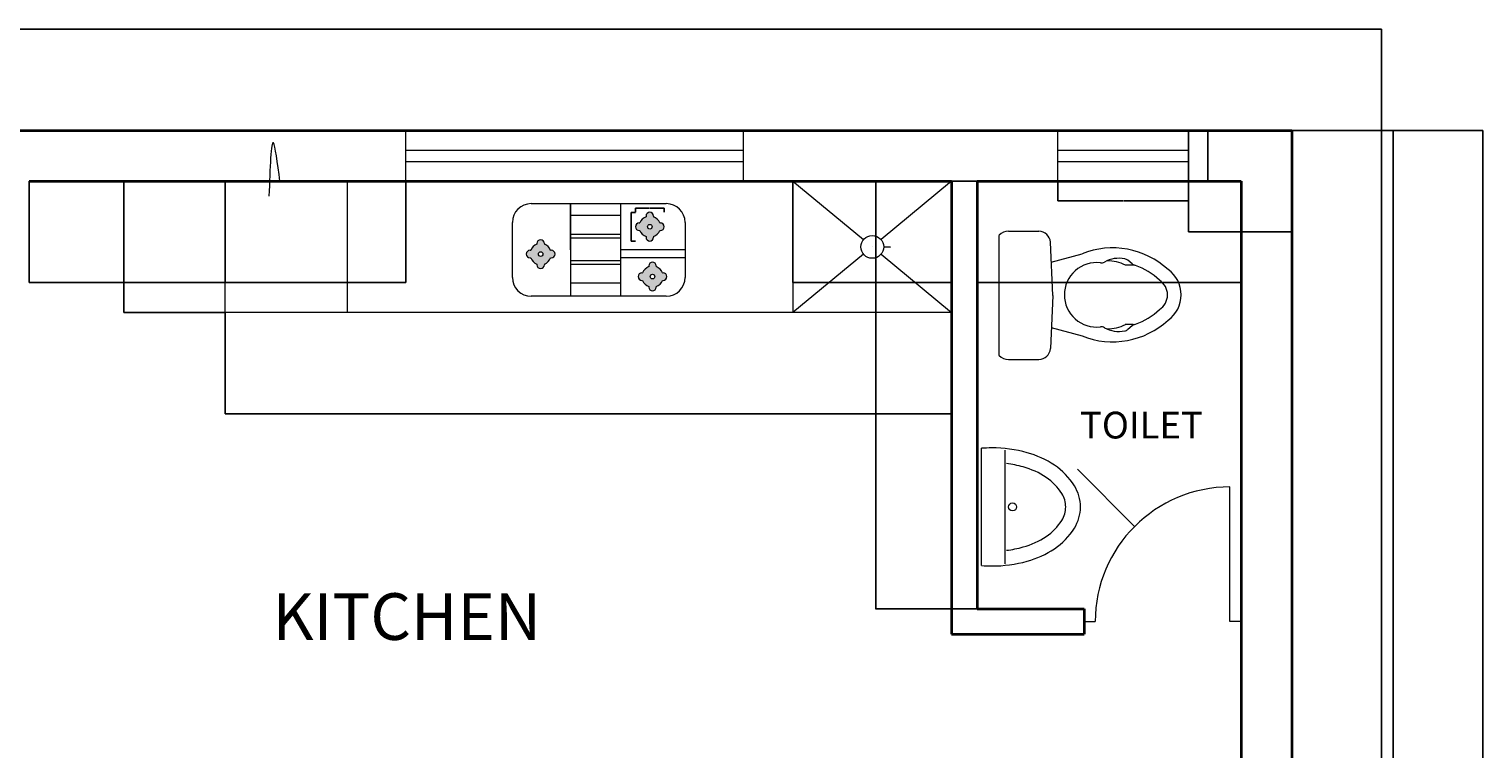
# Model space of a CAD drawing. Units: millimetres. Extents: x 2511 to 24632, y 2213 to 12972.
# Tile 3 of 5: x 6023 to 12605, y 7630 to 10891. Entities that reach past the tile are written whole.
import ezdxf

# ---------------------------------------------------------------- set-up
doc = ezdxf.new("R2010")
doc.units = ezdxf.units.MM
for name, color, linetype, lineweight in [('A-ANNO-DIMS', 2, 'Continuous', 18), ('A-AREA-IDEN', 7, 'Continuous', 20), ('A-EQPM', 4, 'Continuous', 18), ('A-FLOR-CASE', 7, 'Continuous', 18), ('A-FLOR-FIXT', 5, 'Continuous', 18), ('A-WALL', 7, 'Continuous', 35), ('doors', 50, 'Continuous', 18), ('windows', 70, 'Continuous', 18)]:
    doc.layers.add(name, color=color, linetype=linetype, lineweight=lineweight)
doc.styles.get("Standard").update_dxf_attribs({"font": 'arial.ttf'})
doc.dimstyles.get("Standard").update_dxf_attribs({"dimtxt": 0.18, "dimasz": 0.18, "dimexe": 0.18, "dimexo": 0.0625, "dimgap": 0.09, "dimtad": 0, "dimtih": 1, "dimtoh": 1, "dimdec": 4, "dimzin": 0, "dimdsep": 46, "dimtxsty": 'Standard', "dimcen": 0.09, "dimadec": 0, "dimazin": 0, "dimtfac": 1, "dimtdec": 4, "dimtofl": 0, "dimtmove": 0, "dimatfit": 3, "dimfxl": 1, "dimtolj": 1, "dimtzin": 0, "dimarcsym": 0})

# ---------------------------------------------------------------- blocks, each defined once
blk = doc.blocks.new('HOB-BURNER-PLAN')
h = blk.add_hatch(color=256)
h.dxf.hatch_style = 1
h.paths.add_polyline_path([(82.2, 110), (82.2, 113.2, 1), (48.1, 113.2), (48.1, 110, 0.214506), (20.2, 82.2), (17.1, 82.2, 1), (17.1, 48.1), (20.2, 48.1, 0.214506), (48.1, 20.2), (48.1, 17.1, 1), (82.2, 17.1), (82.2, 20.2, 0.214506), (110, 48.1), (113.2, 48.1, 1), (113.2, 82.2), (110, 82.2, 0.214506)])
h.paths.add_polyline_path([(75.5, 65.1, -1), (54.7, 65.1, -1)], flags=16)
for p, q in [((17.1, 82.2), (20.2, 82.2)), ((48.1, 113.2), (48.1, 110)), ((82.2, 113.2), (82.2, 110)), ((110, 82.2), (113.2, 82.2)), ((17.1, 48.1), (20.2, 48.1)), ((48.1, 20.2), (48.1, 17.1)), ((82.2, 20.2), (82.2, 17.1)), ((110, 48.1), (113.2, 48.1))]:
    blk.add_line(p, q)
blk.add_circle((65.1, 65.1), 10.4)
for centre, radius, start, end in [((17.1, 65.1), 17.1, 90, 270), ((65.1, 65.1), 48.1, 110.78637, 159.21363), ((65.1, 113.2), 17.1, 0, 180), ((65.1, 65.1), 48.1, 20.78637, 69.21363), ((113.2, 65.1), 17.1, 270, 90), ((65.1, 65.1), 48.1, 200.78637, 249.21363), ((65.1, 17.1), 17.1, 180, 0), ((65.1, 65.1), 48.1, 290.78637, 339.21363)]:
    blk.add_arc(centre, radius, start, end)
blk = doc.blocks.new('WINDOW-1528-PLAN')
for p, q in [((0, 140), (1528, 140)), ((0, 90), (1528, 90))]:
    blk.add_line(p, q)
blk.add_lwpolyline([(0, 230), (1528, 230), (1528, 0), (0, 0)], close=True)
blk = doc.blocks.new('WINDOW-592-PLAN')
for p, q in [((0, 140), (591.5, 140)), ((0, 90), (591.5, 90))]:
    blk.add_line(p, q)
blk.add_lwpolyline([(0, 230), (591.5, 230), (591.5, 0), (0, 0)], close=True)
blk = doc.blocks.new('*D21')
at = {"layer": 'A-ANNO-DIMS', "color": 0, "lineweight": -2, "transparency": 16777216}
for p, q in [((8768.5, 10060.9), (8768.5, 10080.5)), ((8768.6, 10080.4), (8832.4, 10080.4)), ((8898.5, 10080.4), (8834.7, 10080.4)), ((8898.7, 10060.9), (8898.7, 10080.5))]:
    blk.add_line(p, q, dxfattribs=at)
at = {"layer": 'A-ANNO-DIMS', "color": 0, "transparency": 16777216}
for points in [[(8768.6, 10080.4), (8768.6, 10080.3), (8768.5, 10080.4)], [(8898.5, 10080.4), (8898.5, 10080.3), (8898.7, 10080.4)]]:
    blk.add_solid(points, dxfattribs=at)
at = {"layer": 'Defpoints', "color": 0, "transparency": 16777216}
for p in [(8898.7, 10080.4), (8768.5, 10060.8), (8898.7, 10060.8)]:
    blk.add_point(p, dxfattribs=at)
at = {"layer": 'A-ANNO-DIMS', "color": 0, "transparency": 16777216, "insert": (8833.6, 10080.4), "char_height": 0.18, "attachment_point": 5}
blk.add_mtext('\\A1;BURNER 130 TYP.', dxfattribs=at)
blk = doc.blocks.new('*D22')
at = {"layer": 'A-ANNO-DIMS', "color": 0, "lineweight": -2, "transparency": 16777216}
for p, q in [((8768.4, 10060.8), (8748.7, 10060.8)), ((8748.9, 10060.6), (8748.9, 9995.9)), ((8748.9, 9930.8), (8748.9, 9995.5)), ((8768.4, 9930.6), (8748.7, 9930.6))]:
    blk.add_line(p, q, dxfattribs=at)
at = {"layer": 'A-ANNO-DIMS', "color": 0, "transparency": 16777216}
for points in [[(8748.9, 10060.6), (8749, 10060.6), (8748.9, 10060.8)], [(8748.9, 9930.8), (8749, 9930.8), (8748.9, 9930.6)]]:
    blk.add_solid(points, dxfattribs=at)
at = {"layer": 'Defpoints', "color": 0, "transparency": 16777216}
for p in [(8748.9, 10060.8), (8768.5, 10060.8), (8768.5, 9930.6)]:
    blk.add_point(p, dxfattribs=at)
at = {"layer": 'A-ANNO-DIMS', "color": 0, "transparency": 16777216, "insert": (8748.9, 9995.7), "char_height": 0.18, "attachment_point": 5}
blk.add_mtext('\\A1;130 TYP.', dxfattribs=at)
blk = doc.blocks.new('*D27')
at = {"layer": 'A-ANNO-DIMS', "color": 0, "lineweight": -2, "transparency": 16777216}
for p, q in [((10680.4, 10201.8), (10680.4, 10113)), ((11272, 10201.8), (11272, 10113)), ((10680.6, 10113.1), (10974.8, 10113.1)), ((11271.8, 10113.1), (10977.6, 10113.1))]:
    blk.add_line(p, q, dxfattribs=at)
at = {"layer": 'A-ANNO-DIMS', "color": 0, "transparency": 16777216}
for points in [[(10680.6, 10113.2), (10680.6, 10113.1), (10680.4, 10113.1)], [(11271.8, 10113.2), (11271.8, 10113.1), (11272, 10113.1)]]:
    blk.add_solid(points, dxfattribs=at)
at = {"layer": 'Defpoints', "color": 0, "transparency": 16777216}
for p in [(10680.4, 10201.9), (11272, 10201.9), (11272, 10113.1)]:
    blk.add_point(p, dxfattribs=at)
at = {"layer": 'A-ANNO-DIMS', "color": 0, "transparency": 16777216, "insert": (10976.2, 10113.1), "char_height": 0.18, "attachment_point": 5}
blk.add_mtext('\\A1;WC WINDOW 592 TYP.', dxfattribs=at)
blk = doc.blocks.new('*D28')
at = {"layer": 'A-ANNO-DIMS', "color": 0, "lineweight": -2, "transparency": 16777216}
for p, q in [((11272, 10431.9), (11360.9, 10431.9)), ((11360.7, 10431.7), (11360.7, 10317)), ((11360.7, 10202), (11360.7, 10316.7)), ((11272, 10201.9), (11360.9, 10201.9))]:
    blk.add_line(p, q, dxfattribs=at)
at = {"layer": 'A-ANNO-DIMS', "color": 0, "transparency": 16777216}
for points in [[(11360.7, 10431.7), (11360.7, 10431.7), (11360.7, 10431.9)], [(11360.7, 10202), (11360.7, 10202), (11360.7, 10201.9)]]:
    blk.add_solid(points, dxfattribs=at)
at = {"layer": 'Defpoints', "color": 0, "transparency": 16777216}
for p in [(11272, 10431.9), (11360.7, 10431.9), (11272, 10201.9)]:
    blk.add_point(p, dxfattribs=at)
at = {"layer": 'A-ANNO-DIMS', "color": 0, "transparency": 16777216, "insert": (11360.7, 10316.9), "char_height": 0.18, "attachment_point": 5}
blk.add_mtext('\\A1;230 TYP.', dxfattribs=at)
blk = doc.blocks.new('*D35')
at = {"layer": 'A-ANNO-DIMS', "color": 0, "lineweight": -2, "transparency": 16777216}
for p, q in [((2970.2, 10431.9), (2970.2, 10891)), ((2970.4, 10890.9), (7557.9, 10890.9)), ((12146, 10890.9), (7558.6, 10890.9)), ((12146.2, 7356.9), (12146.2, 10891))]:
    blk.add_line(p, q, dxfattribs=at)
at = {"layer": 'A-ANNO-DIMS', "color": 0, "transparency": 16777216}
for points in [[(2970.4, 10890.9), (2970.4, 10890.8), (2970.2, 10890.9)], [(12146, 10890.9), (12146, 10890.8), (12146.2, 10890.9)]]:
    blk.add_solid(points, dxfattribs=at)
at = {"layer": 'Defpoints', "color": 0, "transparency": 16777216}
for p in [(12146.2, 10890.9), (2970.2, 10431.9), (12146.2, 7356.9)]:
    blk.add_point(p, dxfattribs=at)
at = {"layer": 'A-ANNO-DIMS', "color": 0, "transparency": 16777216, "insert": (7558.2, 10890.9), "char_height": 0.18, "attachment_point": 5}
blk.add_mtext('\\A1;9176', dxfattribs=at)
blk = doc.blocks.new('*D36')
at = {"layer": 'A-ANNO-DIMS', "color": 0, "lineweight": -2, "transparency": 16777216}
for p, q in [((11740.3, 10431.9), (12605.4, 10431.9)), ((12605.2, 10431.7), (12605.2, 6552)), ((12605.2, 2672), (12605.2, 6551.7)), ((9066.3, 2671.9), (12605.4, 2671.9))]:
    blk.add_line(p, q, dxfattribs=at)
at = {"layer": 'A-ANNO-DIMS', "color": 0, "transparency": 16777216}
for points in [[(12605.2, 10431.7), (12605.2, 10431.7), (12605.2, 10431.9)], [(12605.2, 2672), (12605.2, 2672), (12605.2, 2671.9)]]:
    blk.add_solid(points, dxfattribs=at)
at = {"layer": 'Defpoints', "color": 0, "transparency": 16777216}
for p in [(11740.2, 10431.9), (12605.2, 10431.9), (9066.2, 2671.9)]:
    blk.add_point(p, dxfattribs=at)
at = {"layer": 'A-ANNO-DIMS', "color": 0, "transparency": 16777216, "insert": (12605.2, 6551.9), "char_height": 0.18, "attachment_point": 5}
blk.add_mtext('\\A1;7760', dxfattribs=at)
blk = doc.blocks.new('*D50')
at = {"layer": 'A-ANNO-DIMS', "color": 0, "lineweight": -2, "transparency": 16777216}
for p, q in [((6911.1, 9606.7), (6911.1, 9147.6)), ((10200.2, 9606.7), (10200.2, 9147.6)), ((6911.3, 9147.8), (8555.3, 9147.8)), ((10200, 9147.8), (8556, 9147.8))]:
    blk.add_line(p, q, dxfattribs=at)
at = {"layer": 'A-ANNO-DIMS', "color": 0, "transparency": 16777216}
for points in [[(6911.3, 9147.8), (6911.3, 9147.8), (6911.1, 9147.8)], [(10200, 9147.8), (10200, 9147.8), (10200.2, 9147.8)]]:
    blk.add_solid(points, dxfattribs=at)
at = {"layer": 'Defpoints', "color": 0, "transparency": 16777216}
for p in [(6911.1, 9606.8), (10200.2, 9606.8), (6911.1, 9147.8)]:
    blk.add_point(p, dxfattribs=at)
at = {"layer": 'A-ANNO-DIMS', "color": 0, "transparency": 16777216, "insert": (8555.6, 9147.8), "char_height": 0.18, "attachment_point": 5}
blk.add_mtext('\\A1;3289', dxfattribs=at)
blk = doc.blocks.new('*D51')
at = {"layer": 'A-ANNO-DIMS', "color": 0, "lineweight": -2, "transparency": 16777216}
for p, q in [((6911, 10201.9), (6451.9, 10201.9)), ((6452.1, 10201.7), (6452.1, 9904.5)), ((6452.1, 9607), (6452.1, 9904.1)), ((6911, 9606.8), (6451.9, 9606.8))]:
    blk.add_line(p, q, dxfattribs=at)
at = {"layer": 'A-ANNO-DIMS', "color": 0, "transparency": 16777216}
for points in [[(6452, 10201.7), (6452.1, 10201.7), (6452.1, 10201.9)], [(6452, 9607), (6452.1, 9607), (6452.1, 9606.8)]]:
    blk.add_solid(points, dxfattribs=at)
at = {"layer": 'Defpoints', "color": 0, "transparency": 16777216}
for p in [(6452.1, 10201.9), (6911.1, 10201.9), (6911.1, 9606.8)]:
    blk.add_point(p, dxfattribs=at)
at = {"layer": 'A-ANNO-DIMS', "color": 0, "transparency": 16777216, "insert": (6452.1, 9904.3), "char_height": 0.18, "attachment_point": 5}
blk.add_mtext('\\A1;595.1', dxfattribs=at)
blk = doc.blocks.new('*D52')
at = {"layer": 'A-ANNO-DIMS', "color": 0, "lineweight": -2, "transparency": 16777216}
for p, q in [((6023.2, 10201.8), (6023.2, 9742.7)), ((6911.1, 10201.8), (6911.1, 9742.7)), ((6023.4, 9742.9), (6466.8, 9742.9)), ((6910.9, 9742.9), (6467.5, 9742.9))]:
    blk.add_line(p, q, dxfattribs=at)
at = {"layer": 'A-ANNO-DIMS', "color": 0, "transparency": 16777216}
for points in [[(6023.4, 9742.9), (6023.4, 9742.8), (6023.2, 9742.9)], [(6910.9, 9742.9), (6910.9, 9742.8), (6911.1, 9742.9)]]:
    blk.add_solid(points, dxfattribs=at)
at = {"layer": 'Defpoints', "color": 0, "transparency": 16777216}
for p in [(6023.2, 10201.9), (6911.1, 10201.9), (6023.2, 9742.9)]:
    blk.add_point(p, dxfattribs=at)
at = {"layer": 'A-ANNO-DIMS', "color": 0, "transparency": 16777216, "insert": (6467.1, 9742.9), "char_height": 0.18, "attachment_point": 5}
blk.add_mtext('\\A1;887.9', dxfattribs=at)
blk = doc.blocks.new('*D53')
at = {"layer": 'A-ANNO-DIMS', "color": 0, "lineweight": -2, "transparency": 16777216}
for p, q in [((6911.1, 10201.8), (6911.1, 9742.7)), ((7728.6, 10201.8), (7728.6, 9742.7)), ((6911.3, 9742.9), (7319.4, 9742.9)), ((7728.4, 9742.9), (7320.2, 9742.9))]:
    blk.add_line(p, q, dxfattribs=at)
at = {"layer": 'A-ANNO-DIMS', "color": 0, "transparency": 16777216}
for points in [[(6911.3, 9742.9), (6911.3, 9742.8), (6911.1, 9742.9)], [(7728.4, 9742.9), (7728.4, 9742.8), (7728.6, 9742.9)]]:
    blk.add_solid(points, dxfattribs=at)
at = {"layer": 'Defpoints', "color": 0, "transparency": 16777216}
for p in [(6911.1, 10201.9), (7728.6, 10201.9), (6911.1, 9742.9)]:
    blk.add_point(p, dxfattribs=at)
at = {"layer": 'A-ANNO-DIMS', "color": 0, "transparency": 16777216, "insert": (7319.8, 9742.9), "char_height": 0.18, "attachment_point": 5}
blk.add_mtext('\\A1;817.5', dxfattribs=at)
blk = doc.blocks.new('*D54')
at = {"layer": 'A-ANNO-DIMS', "color": 0, "lineweight": -2, "transparency": 16777216}
for p, q in [((9481.2, 10201.8), (9481.2, 9742.7)), ((10200.2, 10201.8), (10200.2, 9742.7)), ((9481.4, 9742.9), (9840.4, 9742.9)), ((10200, 9742.9), (9841, 9742.9))]:
    blk.add_line(p, q, dxfattribs=at)
at = {"layer": 'A-ANNO-DIMS', "color": 0, "transparency": 16777216}
for points in [[(9481.4, 9742.9), (9481.4, 9742.8), (9481.2, 9742.9)], [(10200, 9742.9), (10200, 9742.8), (10200.2, 9742.9)]]:
    blk.add_solid(points, dxfattribs=at)
at = {"layer": 'Defpoints', "color": 0, "transparency": 16777216}
for p in [(9481.2, 10201.9), (10200.2, 10201.9), (9481.2, 9742.9)]:
    blk.add_point(p, dxfattribs=at)
at = {"layer": 'A-ANNO-DIMS', "color": 0, "transparency": 16777216, "insert": (9840.7, 9742.9), "char_height": 0.18, "attachment_point": 5}
blk.add_mtext('\\A1;719', dxfattribs=at)
blk = doc.blocks.new('*D55')
at = {"layer": 'A-ANNO-DIMS', "color": 0, "lineweight": -2, "transparency": 16777216}
for p, q in [((11272, 10431.8), (11272, 9972.7)), ((11740.2, 10431.8), (11740.2, 9972.7)), ((11272.2, 9972.9), (11505.7, 9972.9)), ((11740, 9972.9), (11506.5, 9972.9))]:
    blk.add_line(p, q, dxfattribs=at)
at = {"layer": 'A-ANNO-DIMS', "color": 0, "transparency": 16777216}
for points in [[(11272.2, 9972.9), (11272.2, 9972.8), (11272, 9972.9)], [(11740, 9972.9), (11740, 9972.8), (11740.2, 9972.9)]]:
    blk.add_solid(points, dxfattribs=at)
at = {"layer": 'Defpoints', "color": 0, "transparency": 16777216}
for p in [(11272, 10431.9), (11740.2, 10431.9), (11272, 9972.9)]:
    blk.add_point(p, dxfattribs=at)
at = {"layer": 'A-ANNO-DIMS', "color": 0, "transparency": 16777216, "insert": (11506.1, 9972.9), "char_height": 0.18, "attachment_point": 5}
blk.add_mtext('\\A1;468.2', dxfattribs=at)
blk = doc.blocks.new('*D56')
at = {"layer": 'A-ANNO-DIMS', "color": 0, "lineweight": -2, "transparency": 16777216}
for p, q in [((10315.2, 10201.8), (10315.2, 9742.7)), ((11510.2, 10201.8), (11510.2, 9742.7)), ((10315.4, 9742.9), (10912.4, 9742.9)), ((11510, 9742.9), (10913.1, 9742.9))]:
    blk.add_line(p, q, dxfattribs=at)
at = {"layer": 'A-ANNO-DIMS', "color": 0, "transparency": 16777216}
for points in [[(10315.4, 9742.9), (10315.4, 9742.8), (10315.2, 9742.9)], [(11510, 9742.9), (11510, 9742.8), (11510.2, 9742.9)]]:
    blk.add_solid(points, dxfattribs=at)
at = {"layer": 'Defpoints', "color": 0, "transparency": 16777216}
for p in [(10315.2, 10201.9), (11510.2, 10201.9), (10315.2, 9742.9)]:
    blk.add_point(p, dxfattribs=at)
at = {"layer": 'A-ANNO-DIMS', "color": 0, "transparency": 16777216, "insert": (10912.7, 9742.9), "char_height": 0.18, "attachment_point": 5}
blk.add_mtext('\\A1;1195', dxfattribs=at)
blk = doc.blocks.new('*D57')
at = {"layer": 'A-ANNO-DIMS', "color": 0, "lineweight": -2, "transparency": 16777216}
for p, q in [((10315.2, 10201.9), (9856, 10201.9)), ((9856.2, 10201.7), (9856.2, 9233.4)), ((9856.2, 8264.7), (9856.2, 9233)), ((10315.2, 8264.5), (9856, 8264.5))]:
    blk.add_line(p, q, dxfattribs=at)
at = {"layer": 'A-ANNO-DIMS', "color": 0, "transparency": 16777216}
for points in [[(9856.2, 10201.7), (9856.2, 10201.7), (9856.2, 10201.9)], [(9856.2, 8264.7), (9856.2, 8264.7), (9856.2, 8264.5)]]:
    blk.add_solid(points, dxfattribs=at)
at = {"layer": 'Defpoints', "color": 0, "transparency": 16777216}
for p in [(9856.2, 10201.9), (10315.2, 10201.9), (10315.2, 8264.5)]:
    blk.add_point(p, dxfattribs=at)
at = {"layer": 'A-ANNO-DIMS', "color": 0, "transparency": 16777216, "insert": (9856.2, 9233.2), "char_height": 0.18, "attachment_point": 5}
blk.add_mtext('\\A1;1937.4', dxfattribs=at)
blk = doc.blocks.new('*D59')
at = {"layer": 'A-ANNO-DIMS', "color": 0, "lineweight": -2, "transparency": 16777216}
for p, q in [((11740.3, 10431.9), (12199.4, 10431.9)), ((12199.2, 10431.7), (12199.2, 8779.5)), ((12199.2, 7127), (12199.2, 8779.2)), ((11740.3, 7126.9), (12199.4, 7126.9))]:
    blk.add_line(p, q, dxfattribs=at)
at = {"layer": 'A-ANNO-DIMS', "color": 0, "transparency": 16777216}
for points in [[(12199.2, 10431.7), (12199.2, 10431.7), (12199.2, 10431.9)], [(12199.2, 7127), (12199.2, 7127), (12199.2, 7126.9)]]:
    blk.add_solid(points, dxfattribs=at)
at = {"layer": 'Defpoints', "color": 0, "transparency": 16777216}
for p in [(11740.2, 10431.9), (11740.2, 7126.9), (12199.2, 7126.9)]:
    blk.add_point(p, dxfattribs=at)
at = {"layer": 'A-ANNO-DIMS', "color": 0, "transparency": 16777216, "insert": (12199.2, 8779.4), "char_height": 0.18, "attachment_point": 5}
blk.add_mtext('\\A1;3305', dxfattribs=at)
blk = doc.blocks.new('*D96')
at = {"layer": 'A-ANNO-DIMS', "color": 0, "lineweight": -2, "transparency": 16777216}
for p, q in [((9840.6, 9904.3), (9840.8, 9904.3)), ((9840.7, 9904.2), (9840.7, 9904.4)), ((9923.4, 9903.8), (9892.5, 9904))]:
    blk.add_line(p, q, dxfattribs=at)
at = {"layer": 'A-ANNO-DIMS', "color": 0, "transparency": 16777216}
blk.add_solid([(9892.5, 9904), (9892.5, 9904), (9892.4, 9904)], dxfattribs=at)
at = {"layer": 'Defpoints', "color": 0, "transparency": 16777216}
for p in [(9789, 9904.7), (9892.4, 9904)]:
    blk.add_point(p, dxfattribs=at)
at = {"layer": 'A-ANNO-DIMS', "color": 0, "transparency": 16777216, "insert": (9923.9, 9903.8), "char_height": 0.18, "attachment_point": 5}
blk.add_mtext('\\A1;∅103.33', dxfattribs=at)
blk = doc.blocks.new('*D101')
at = {"layer": 'A-ANNO-DIMS', "color": 0, "lineweight": -2, "transparency": 16777216}
for p, q in [((10769.7, 8897), (10769.9, 8897)), ((10769.9, 8897), (11028.6, 8638.4)), ((11460.1, 8207), (11460.3, 8207)), ((11460.2, 8206.9), (11460.2, 8207.1))]:
    blk.add_line(p, q, dxfattribs=at)
at = {"layer": 'A-ANNO-DIMS', "color": 0, "transparency": 16777216}
blk.add_solid([(11028.7, 8638.4), (11028.6, 8638.3), (11028.8, 8638.2)], dxfattribs=at)
at = {"layer": 'Defpoints', "color": 0, "transparency": 16777216}
for p in [(11028.8, 8638.2), (11460.2, 8207)]:
    blk.add_point(p, dxfattribs=at)
at = {"layer": 'A-ANNO-DIMS', "color": 0, "transparency": 16777216, "insert": (10769.4, 8897), "char_height": 0.18, "attachment_point": 5}
blk.add_mtext('\\A1;R610', dxfattribs=at)

msp = doc.modelspace()

# ---------------------------------------------------------------- linework, layer by layer
at = {"layer": 'A-EQPM'}
for p, q in [((8296.911, 10100.301), (8908.113, 10100.301)), ((8474.03, 9890.438), (8474.03, 10100.301)), ((8474.03, 10100.301), (8474.03, 9680.576)), ((8701.627, 10100.301), (8701.627, 9680.576)), ((8211.637, 9765.85), (8211.637, 10015.027)), ((8474.03, 10047.835), (8701.627, 10047.835)), ((8993.387, 10015.027), (8993.387, 9765.85)), ((8474.03, 9962.561), (8701.627, 9962.561)), ((8474.03, 9945.506), (8701.627, 9945.506)), ((8993.387, 9890.438), (8701.627, 9890.438)), ((8474.03, 9843.178), (8701.627, 9843.178)), ((8474.03, 9826.123), (8701.627, 9826.123)), ((8701.627, 9856.329), (8993.387, 9856.329)), ((8908.113, 9680.576), (8296.911, 9680.576)), ((8474.03, 9740.849), (8701.627, 9740.849))]:
    msp.add_line(p, q, dxfattribs=at)
for centre, start, end in [((8296.911, 10015.027), 90, 180), ((8908.113, 10015.027), 0, 90), ((8296.911, 9765.85), 180, 270), ((8908.113, 9765.85), 270, 0)]:
    msp.add_arc(centre, 85.274, start, end, dxfattribs=at)
at = {"layer": 'A-FLOR-CASE'}
for p, q in [((7463.966, 10201.864), (7463.966, 9606.794)), ((9481.195, 10201.864), (9481.195, 9606.794))]:
    msp.add_line(p, q, dxfattribs=at)
msp.add_lwpolyline([(6911.074, 10201.864), (10200.215, 10201.864), (10200.215, 9606.794), (6911.074, 9606.794)], close=True, dxfattribs=at)
at = {"layer": 'A-FLOR-FIXT'}
for p, q in [((9481.195, 10201.864), (9800.902, 9937.27)), ((10200.215, 10201.864), (9880.507, 9937.27)), ((9800.902, 9871.388), (9481.195, 9606.794)), ((9880.507, 9871.388), (10200.215, 9606.794)), ((10334.863, 8460.732), (10334.863, 8991.932)), ((10441.908, 8468.588), (10441.908, 8984.077))]:
    msp.add_line(p, q, dxfattribs=at)
at = {"layer": 'A-FLOR-FIXT', "ltscale": 20}
for p, q in [((10413.941, 9952.477), (10413.941, 9416.941)), ((10456.824, 9975.056), (10595.083, 9975.056)), ((10657.782, 9684.709), (10646.952, 9925.467)), ((10651.013, 9835.172), (10790.548, 9873.204)), ((11022.229, 9821.776), (10986.239, 9821.776)), ((11017.43, 9827.388), (10998.079, 9843.626)), ((10657.782, 9684.709), (10646.952, 9443.95)), ((11022.229, 9552.296), (10986.239, 9552.296)), ((11017.43, 9546.685), (10998.079, 9530.447)), ((10651.22, 9538.845), (10790.548, 9500.868)), ((10456.824, 9394.361), (10595.083, 9394.361))]:
    msp.add_line(p, q, dxfattribs=at)
at = {"layer": 'A-FLOR-FIXT'}
for points in [[(10783.239, 8726.332, 0.13988915), (10755.814, 8822.44, 0.10711811), (10665.734, 8915.455, 0.07981249), (10541.677, 8972.157, 0.06745904), (10382.05, 8993.792, 0.01969394), (10334.863, 8991.932, 0.02043933)], [(10716.374, 8726.332, 0.13988915), (10699.019, 8787.152, 0.10711811), (10628.644, 8859.82, 0.07981249), (10523.879, 8907.704, 0.03606883), (10448.594, 8922.755, 0.02217222)], [(10334.863, 8460.732, 0.01969394), (10382.05, 8458.873, 0.06745904), (10541.677, 8480.508, 0.07981249), (10665.734, 8537.21, 0.10711811), (10755.814, 8630.225, 0.13988915), (10783.239, 8726.332, 0.13988915)], [(10448.594, 8529.909, 0.03606883), (10523.879, 8544.96, 0.07981249), (10628.644, 8592.845, 0.10711811), (10699.019, 8665.513, 0.13988915), (10716.374, 8726.332, 0.13988915)]]:
    msp.add_lwpolyline(points, format="xyb", dxfattribs=at)
for centre, radius in [((9840.705, 9904.329), 51.665), ((10475.712, 8726.332), 18.177)]:
    msp.add_circle(centre, radius, dxfattribs=at)
at = {"layer": 'A-FLOR-FIXT', "ltscale": 20}
for centre, radius, start, end in [((10421.21, 9952.477), 7.269, 136.5268908, 180), ((10456.824, 9918.712), 56.343, 90, 136.5268908), ((10595.083, 9923.134), 51.922, 2.5755369, 90), ((10928.527, 9528.1), 371.666, 47.4134513, 111.7924053), ((10856.568, 9687.036), 146.159, 83.3522633, 180), ((10877.064, 9862.896), 30.891, 263.3522633, 298.574155), ((10958.328, 9713.688), 139.011, 79.3968296, 118.574155), ((10904.526, 9655.899), 185.348, 63.5020229, 90.4521643), ((10978.222, 9819.961), 30.891, 50, 79.3968296), ((11037.287, 9851.052), 30.891, 230, 251.3881237), ((11022.229, 9790.885), 30.891, 70.3751037, 90), ((10928.527, 9528.1), 309.883, 46.6119806, 70.3751037), ((11098.853, 9687.036), 78.743, 0, 57.2973839), ((11098.853, 9687.036), 140.525, 0, 54.7114749), ((10856.568, 9687.036), 146.159, 180, 276.6477367), ((11098.853, 9687.036), 78.743, 302.7026161, 0), ((11098.853, 9687.036), 140.525, 305.2885251, 0), ((10928.527, 9845.973), 309.883, 289.6248963, 313.3880194), ((10928.527, 9845.973), 371.666, 248.2075947, 312.5865487), ((10904.526, 9718.174), 185.348, 269.5478357, 296.4979771), ((11037.287, 9523.02), 30.891, 108.6118763, 130), ((11022.229, 9583.188), 30.891, 270, 289.6248963), ((10877.064, 9511.177), 30.891, 61.425845, 96.6477367), ((10958.328, 9660.385), 139.011, 241.425845, 280.6031704), ((10978.222, 9554.111), 30.891, 280.6031704, 310), ((10421.21, 9416.941), 7.269, 180, 223.4731092), ((10595.083, 9446.283), 51.922, 270, 357.4244631), ((10456.824, 9450.705), 56.343, 223.4731092, 270)]:
    msp.add_arc(centre, radius, start, end, dxfattribs=at)
at = {"layer": 'A-FLOR-FIXT'}
msp.add_open_spline([(7159.042, 10201.864), (7147.981, 10284.165), (7121.704, 10479.679), (7113.949, 10260.759), (7109.459, 10133.992)], degree=3, knots=[0, 0, 0, 0, 176.02533968, 418.16498855, 418.16498855, 418.16498855, 418.16498855], dxfattribs=at)
at = {"layer": 'A-WALL'}
for p, q in [((2970.215, 10431.864), (11740.215, 10431.864)), ((11740.215, 10431.864), (11740.215, 7126.864)), ((6023.215, 10201.864), (10200.215, 10201.864)), ((10200.215, 10201.864), (10200.215, 8149.499)), ((10315.215, 10201.864), (10315.215, 8264.499)), ((10315.215, 10201.864), (11510.215, 10201.864)), ((11510.215, 10201.864), (11510.215, 7241.864)), ((10315.215, 8264.499), (10800.215, 8264.499)), ((10800.215, 8264.499), (10800.215, 8149.499)), ((10200.215, 8149.499), (10800.215, 8149.499))]:
    msp.add_line(p, q, dxfattribs=at)
at = {"layer": 'doors'}
for p, q in [((11460.215, 8206.999), (11460.215, 8816.999)), ((10800.215, 8206.999), (10850.215, 8206.999)), ((11510.215, 8206.999), (11460.215, 8206.999))]:
    msp.add_line(p, q, dxfattribs=at)
msp.add_arc((11460.215, 8206.999), 610, 90, 180, dxfattribs=at)

# ---------------------------------------------------------------- block references
at = {"layer": 'A-EQPM'}
for p in [(8768.463, 9930.603), (8274.272, 9806.559), (8780.728, 9704.747)]:
    msp.add_blockref('HOB-BURNER-PLAN', p, dxfattribs=at)
at = {"layer": 'windows'}
for name, p in [('WINDOW-1528-PLAN', (7728.602, 10201.864)), ('WINDOW-592-PLAN', (10680.436, 10201.864))]:
    msp.add_blockref(name, p, dxfattribs=at)

# ---------------------------------------------------------------- texts
at = {"layer": 'A-AREA-IDEN', "attachment_point": 1}
for s, width, gutter_width, insert, char_height in [('{\\fArial|b1|i0|c0|p34;TOILET}', 618.99213, 605.738, (10781.279, 9157.636), 121.14764), ('{\\fArial|b1|i0|c0|p34;KITCHEN}', 1956.1379, 1056.928, (7124.976, 8335.434), 211.38565)]:
    msp.add_mtext_dynamic_manual_height_columns(s, width=width, gutter_width=gutter_width, heights=[0], dxfattribs=dict(at, insert=insert, char_height=char_height))

# ---------------------------------------------------------------- dimensions: what is measured, and where the dimension line sits
at = {"layer": 'A-ANNO-DIMS'}
dim = msp.add_linear_dim(base=(12146.215, 10890.864), p1=(2970.215, 10431.864), p2=(12146.215, 7356.864), dimstyle='Standard', override={"dimdec": 0, "dimlfac": 1, "dimrnd": 0, "dimzin": 0, "dimdsep": 46, "dimlunit": 2}, dxfattribs=at)
dim.commit()
dim.dimension.update_dxf_attribs({"geometry": '*D35', "text_midpoint": (7558.215, 10890.864)})
for base, p1, p2, angle, override, picture, middle in [((12605.215, 10431.864), (9066.215, 2671.864), (11740.215, 10431.864), 90, {"dimdec": 0, "dimlfac": 1, "dimrnd": 0, "dimzin": 0, "dimdsep": 46, "dimlunit": 2}, '*D36', (12605.215, 6551.864)), ((11271.984, 9972.864), (11740.215, 10431.864), (11271.984, 10431.864), 180, {"dimdec": 1, "dimlfac": 1, "dimrnd": 0, "dimzin": 0, "dimdsep": 46, "dimlunit": 2}, '*D55', (11506.1, 9972.864)), ((12199.215, 7126.864), (11740.215, 10431.864), (11740.215, 7126.864), 270, {"dimdec": 0, "dimlfac": 1, "dimrnd": 0, "dimzin": 0, "dimdsep": 46, "dimlunit": 2}, '*D59', (12199.215, 8779.364)), ((6023.215, 9742.864), (6911.074, 10201.864), (6023.215, 10201.864), 180, {"dimdec": 1, "dimlfac": 1, "dimrnd": 0, "dimzin": 0, "dimdsep": 46, "dimlunit": 2}, '*D52', (6467.144, 9742.864)), ((6452.074, 10201.864), (6911.074, 9606.794), (6911.074, 10201.864), 90, {"dimdec": 1, "dimlfac": 1, "dimrnd": 0, "dimzin": 0, "dimdsep": 46, "dimlunit": 2}, '*D51', (6452.074, 9904.329)), ((6911.074, 9742.864), (7728.601, 10201.864), (6911.074, 10201.864), 180, {"dimdec": 1, "dimlfac": 1, "dimrnd": 0, "dimzin": 0, "dimdsep": 46, "dimlunit": 2}, '*D53', (7319.838, 9742.864)), ((9481.195, 9742.864), (10200.215, 10201.864), (9481.195, 10201.864), 180, {"dimdec": 0, "dimlfac": 1, "dimrnd": 0, "dimzin": 0, "dimdsep": 46, "dimlunit": 2}, '*D54', (9840.705, 9742.864)), ((9856.215, 10201.864), (10315.215, 8264.499), (10315.215, 10201.864), 90, {"dimdec": 1, "dimlfac": 1, "dimrnd": 0, "dimzin": 0, "dimdsep": 46, "dimlunit": 2}, '*D57', (9856.215, 9233.181)), ((10315.215, 9742.864), (11510.215, 10201.864), (10315.215, 10201.864), 180, {"dimdec": 0, "dimlfac": 1, "dimrnd": 0, "dimzin": 0, "dimdsep": 46, "dimlunit": 2}, '*D56', (10912.715, 9742.864)), ((6911.074, 9147.794), (10200.215, 9606.794), (6911.074, 9606.794), 180, {"dimdec": 0, "dimlfac": 1, "dimrnd": 0, "dimzin": 0, "dimdsep": 46, "dimlunit": 2}, '*D50', (8555.644, 9147.794))]:
    dim = msp.add_linear_dim(base=base, p1=p1, p2=p2, angle=angle, dimstyle='Standard', override=override, dxfattribs=at)
    dim.commit()
    dim.dimension.update_dxf_attribs({"geometry": picture, "text_midpoint": middle})
for base, p1, p2, picture, middle in [((11360.717, 10431.864), (11271.984, 10201.864), (11271.984, 10431.864), '*D28', (11360.717, 10316.864)), ((8748.929, 10060.827), (8768.463, 9930.603), (8768.463, 10060.827), '*D22', (8748.929, 9995.715))]:
    dim = msp.add_linear_dim(base=base, p1=p1, p2=p2, angle=90, text='<> TYP.', dimstyle='Standard', override={"dimdec": 0, "dimlfac": 1, "dimrnd": 0, "dimzin": 0, "dimdsep": 46, "dimlunit": 2}, dxfattribs=at)
    dim.commit()
    dim.dimension.update_dxf_attribs({"geometry": picture, "text_midpoint": middle})
for base, p1, p2, text, picture, middle in [((11271.984, 10113.131), (10680.436, 10201.864), (11271.984, 10201.864), 'WC WINDOW <> TYP.', '*D27', (10976.21, 10113.131)), ((8898.687, 10080.361), (8768.463, 10060.827), (8898.687, 10060.827), 'BURNER <> TYP.', '*D21', (8833.575, 10080.361))]:
    dim = msp.add_linear_dim(base=base, p1=p1, p2=p2, text=text, dimstyle='Standard', override={"dimdec": 0, "dimlfac": 1, "dimrnd": 0, "dimzin": 0, "dimdsep": 46, "dimlunit": 2}, dxfattribs=at)
    dim.commit()
    dim.dimension.update_dxf_attribs({"geometry": picture, "text_midpoint": middle})
dim = msp.add_diameter_dim_2p(p1=(9789.04, 9904.654), p2=(9892.369, 9904.004), dimstyle='Standard', override={"dimdec": 2, "dimlfac": 1, "dimrnd": 0, "dimzin": 0, "dimdsep": 46, "dimlunit": 2}, dxfattribs=at)
dim.commit()
dim.dimension.update_dxf_attribs({"geometry": '*D96', "text_midpoint": (9923.368, 9903.809), "dimtype": 163})
dim = msp.add_radius_dim(center=(11460.215, 8206.999), mpoint=(11028.773, 8638.227), dimstyle='Standard', override={"dimdec": 0, "dimlfac": 1, "dimrnd": 0, "dimzin": 0, "dimdsep": 46, "dimlunit": 2}, dxfattribs=at)
dim.commit()
dim.dimension.update_dxf_attribs({"geometry": '*D101', "text_midpoint": (10769.353, 8896.965), "dimtype": 164})

doc.saveas('drawing.dxf')
